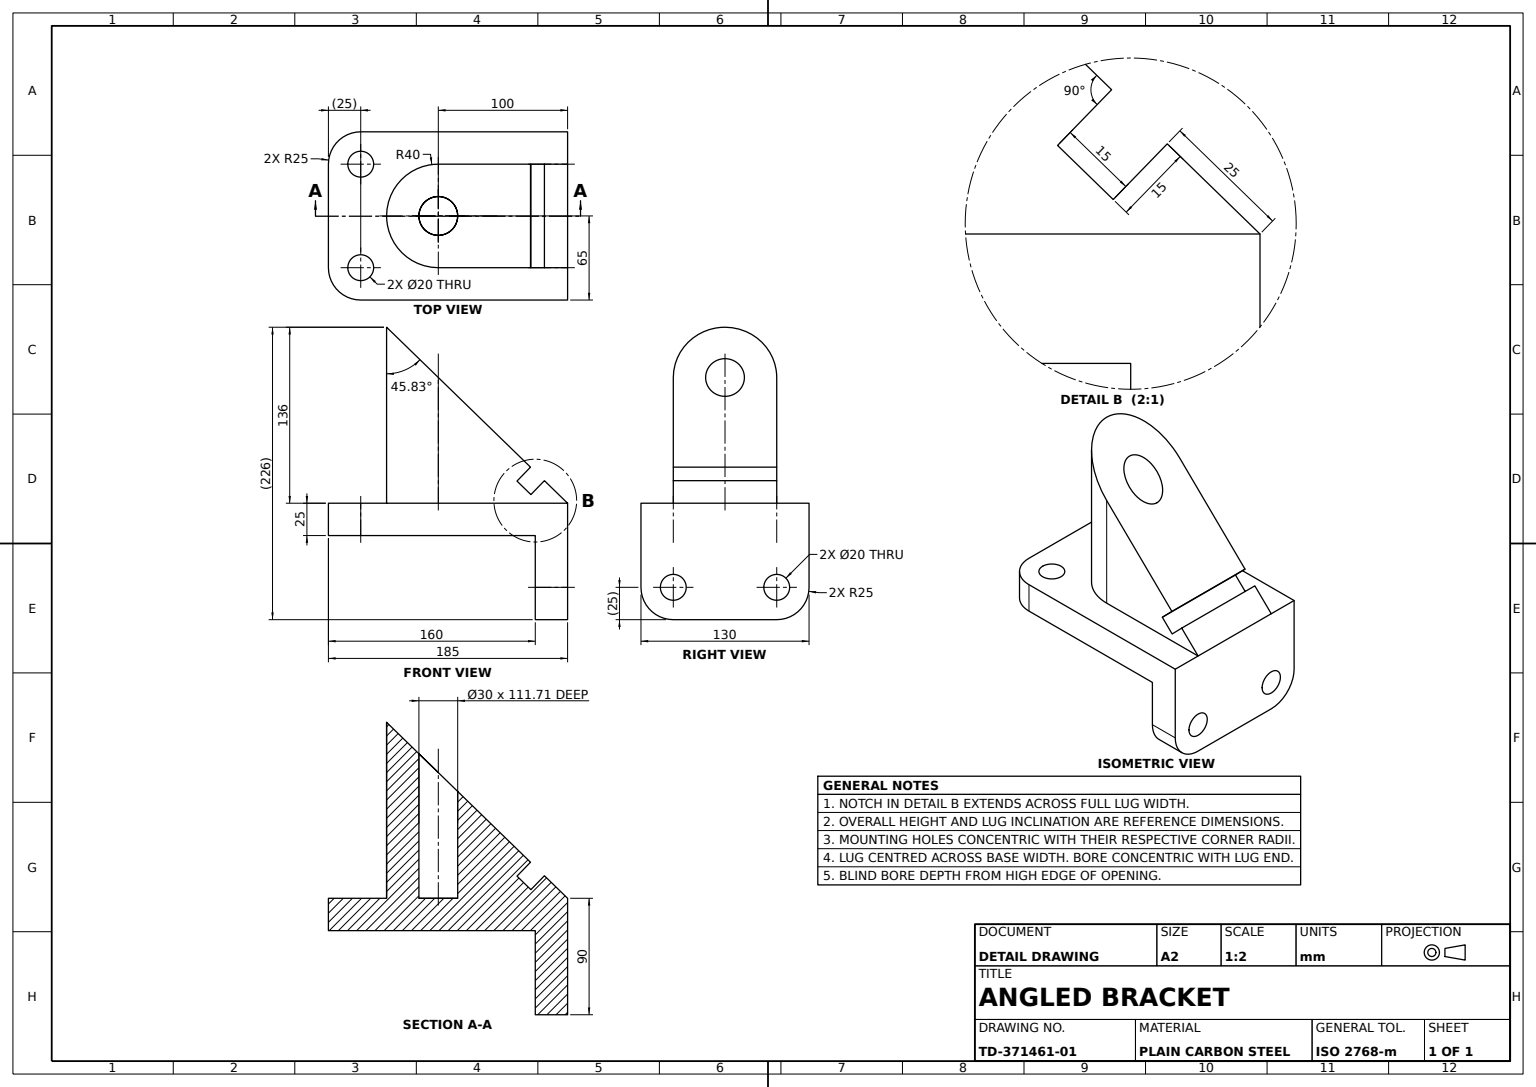
from build123d import *

# Parameters (mm, degrees)
BASE_PLATE_SKETCH_R      = 10
BASE_PLATE_DEPTH         = 25
FLANGE_SKETCH_W          = 130
FLANGE_SKETCH_H          = 25
FLANGE_DEPTH             = 160
FLANGE_PROFILE_CUT_DEPTH = 160
HOLES_SKETCH_R           = 10
HOLES_CUT_DEPTH          = 160
LUG_SKETCH_R             = 15
LUG_DEPTH                = 136
LUG_45DEG_TRIM_DEPTH     = 136
LUG_NOTCH_DEPTH          = 136


with BuildPart() as part:
    # Base Plate Sketch → Base Plate (new body)
    with BuildSketch(Plane.XY):
        with BuildLine():
            Line((-69.89539749, 0), (60.10460251, 0))
            Line((60.10460251, 0), (60.10460251, -65))
            ThreePointArc((60.10460251, -65), (52.78227204, -82.67766953), (35.10460251, -90))
            Line((35.10460251, -90), (-44.89539749, -90))
            ThreePointArc((-44.89539749, -90), (-62.573067019, -82.67766953), (-69.89539749, -65))
            Line((-69.89539749, -65), (-69.89539749, 0))
        make_face()
        with Locations((-44.89539749, -65)):
            Circle(BASE_PLATE_SKETCH_R, mode=Mode.SUBTRACT)
        with Locations((35.10460251, -65)):
            Circle(BASE_PLATE_SKETCH_R, mode=Mode.SUBTRACT)
    extrude(amount=BASE_PLATE_DEPTH)

    # Flange Sketch → Flange (add)
    with BuildSketch(Plane(origin=(0, 0, 0), x_dir=(-1, 0, 0), z_dir=(0, 0, -1))):
        with Locations((4.89539749, -12.5)):
            Rectangle(FLANGE_SKETCH_W, FLANGE_SKETCH_H)
    extrude(amount=FLANGE_DEPTH)

    # Flange Profile Cut Sketch → Flange Profile Cut (cut)
    with BuildSketch(Plane(origin=(0, 0, 0), x_dir=(1, 0, 0), z_dir=(0, 1, 0))):
        with BuildLine():
            Line((60.10460251, 160), (35.10460251, 160))
            ThreePointArc((35.10460251, 160), (52.78227204, 152.67766953), (60.10460251, 135))
            Line((60.10460251, 135), (60.10460251, 160))
        make_face()
        with BuildLine():
            ThreePointArc((-69.89539749, 135), (-62.573067019, 152.67766953), (-44.89539749, 160))
            Line((-44.89539749, 160), (-69.89539749, 160))
            Line((-69.89539749, 160), (-69.89539749, 135))
        make_face()
    extrude(amount=-FLANGE_PROFILE_CUT_DEPTH, mode=Mode.SUBTRACT)

    # Holes Sketch → Holes Cut (cut)
    with BuildSketch(Plane(origin=(0, 0, 0), x_dir=(1, 0, 0), z_dir=(0, 1, 0))):
        with Locations(Location((-44.89539749, 135, 0), (0, 0, 270))):
            Circle(HOLES_SKETCH_R)
        with Locations(Location((35.10460251, 135, 0), (0, 0, 270))):
            Circle(HOLES_SKETCH_R)
    extrude(amount=-HOLES_CUT_DEPTH, mode=Mode.SUBTRACT)

    # Lug Sketch → Lug (add)
    with BuildSketch(Plane(origin=(0, 0, 0), x_dir=(1, 0, 0), z_dir=(0, 1, 0))):
        with BuildLine():
            Line((-44.89539749, -25), (35.10460251, -25))
            Line((35.10460251, -25), (35.10460251, 75))
            ThreePointArc((35.10460251, 75), (-4.89539749, 115), (-44.89539749, 75))
            Line((-44.89539749, 75), (-44.89539749, -25))
        make_face()
        with Locations(Location((-4.89539749, 75, 0), (0, 0, 270))):
            Circle(LUG_SKETCH_R, mode=Mode.SUBTRACT)
    extrude(amount=LUG_DEPTH)

    # Lug 45deg Trim Sketch → Lug 45deg Trim (cut)
    with BuildSketch(Plane(origin=(35.10460251, 0, 0), x_dir=(0, 0, -1), z_dir=(1, 0, 0))):
        Polygon((-25, 0), (-25, 136), (115, 136), align=None)
    extrude(amount=-LUG_45DEG_TRIM_DEPTH, mode=Mode.SUBTRACT)

    # Lug Notch Sketch → Lug Notch (cut)
    with BuildSketch(Plane(origin=(35.10460251, 0, 0), x_dir=(0, 0, -1), z_dir=(1, 0, 0))):
        Polygon((-7.068015479, 17.419642107), (3.691175234, 27.871427371), (14.142960498, 17.112236658), (3.383769785, 6.660451394), align=None)
    extrude(amount=-LUG_NOTCH_DEPTH, mode=Mode.SUBTRACT)


solid = part.part
